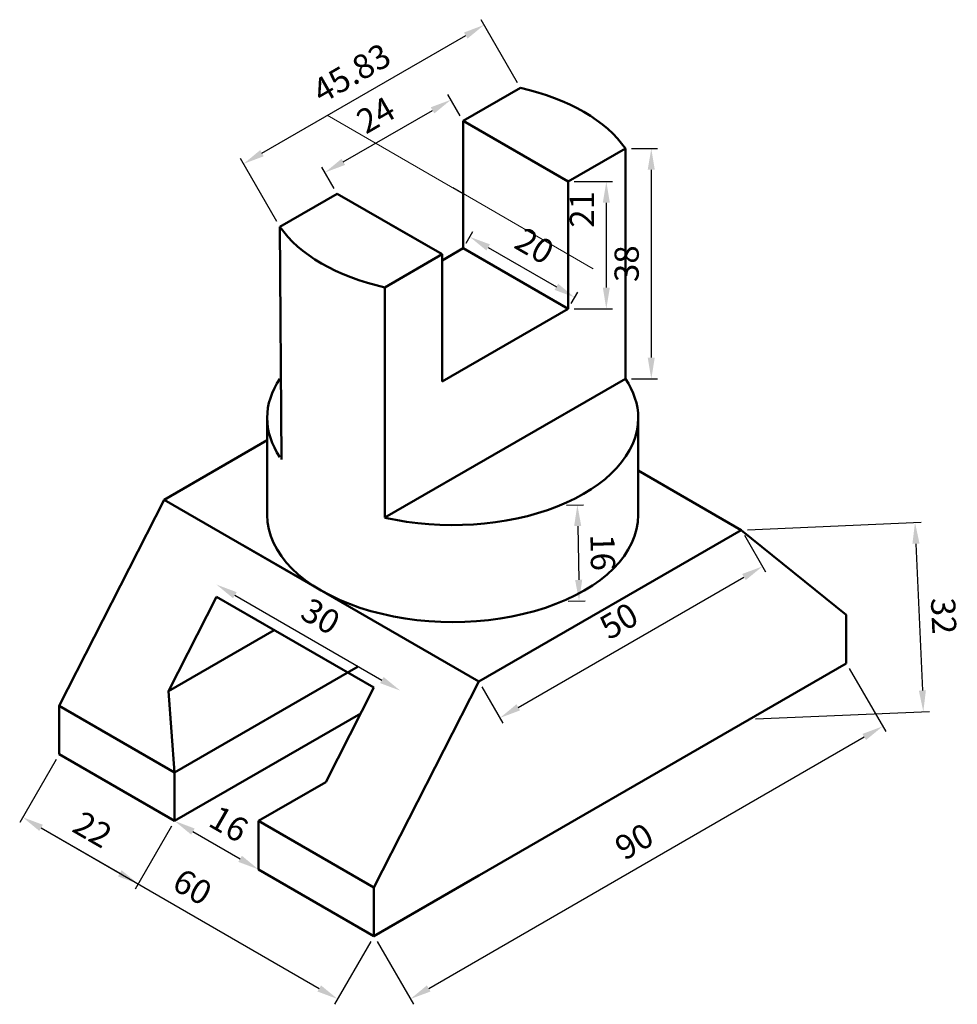
# Model space of a CAD drawing. Units: millimetres. Extents: x 3187 to 3342, y 774 to 936.
import ezdxf

# ---------------------------------------------------------------- set-up
doc = ezdxf.new("R2010")
doc.units = ezdxf.units.MM
doc.linetypes.add('CENTER', pattern=[50.8, 31.75, -6.35, 6.35, -6.35])
for name, color, linetype, lineweight in [('M-CNTR', 4, 'CENTER', 18), ('M-DIMS', 3, 'Continuous', 25), ('M-OUTL', 7, 'Continuous', 50)]:
    doc.layers.add(name, color=color, linetype=linetype, lineweight=lineweight)
doc.styles.get("Standard").update_dxf_attribs({"font": 'arial.ttf'})
doc.dimstyles.new('AM_ISO$0', dxfattribs={"dimtxt": 4, "dimasz": 3.5, "dimexe": 1, "dimexo": 1, "dimgap": 1.5, "dimtad": 1, "dimdsep": 46, "dimtxsty": 'Standard', "dimcen": 0, "dimclrd": 256, "dimclre": 256, "dimclrt": 2, "dimadec": 0, "dimazin": 2, "dimtp": 0.1, "dimtm": 0.1, "dimtfac": 0.71, "dimtmove": 0, "dimatfit": 3, "dimfxl": 1, "dimlwd": -1, "dimlwe": -1, "dimarcsym": 1})

# ---------------------------------------------------------------- blocks, each defined once
blk = doc.blocks.new('*D3')
at = {"layer": 'Defpoints', "color": 0, "transparency": 16777216}
for p in [(3323.73, 829.92), (3329.73, 819.53), (3245.79, 784.92)]:
    blk.add_point(p, dxfattribs=at)
at = {"layer": 'M-DIMS', "color": 0, "linetype": 'ByBlock', "transparency": 16777216}
for p, q in [((3324.23, 829.05), (3330.23, 818.66)), ((3254.82, 776.28), (3326.7, 817.78)), ((3246.29, 784.05), (3252.29, 773.66))]:
    blk.add_line(p, q, dxfattribs=at)
at = {"layer": 'M-DIMS', "color": 0, "transparency": 16777216}
for points in [[(3326.4, 818.28), (3326.99, 817.27), (3329.73, 819.53)], [(3254.52, 776.78), (3255.11, 775.77), (3251.79, 774.53)]]:
    blk.add_solid(points, dxfattribs=at)
at = {"layer": 'M-DIMS', "color": 0, "transparency": 16777216, "insert": (3288.99, 800.09), "char_height": 4, "attachment_point": 5, "rotation": 30}
blk.add_mtext('90', dxfattribs=at)
blk = doc.blocks.new('*D4')
at = {"layer": 'Defpoints', "color": 0, "transparency": 16777216}
for p in [(3306.41, 851.92), (3309.88, 845.91), (3263.11, 826.92)]:
    blk.add_point(p, dxfattribs=at)
at = {"layer": 'M-DIMS', "color": 0, "linetype": 'ByBlock', "transparency": 16777216}
for p, q in [((3306.91, 851.05), (3310.38, 845.05)), ((3269.6, 822.66), (3306.84, 844.16)), ((3263.61, 826.05), (3267.07, 820.05))]:
    blk.add_line(p, q, dxfattribs=at)
at = {"layer": 'M-DIMS', "color": 0, "transparency": 16777216}
for points in [[(3306.55, 844.67), (3307.14, 843.66), (3309.88, 845.91)], [(3269.31, 823.17), (3269.9, 822.16), (3266.57, 820.91)]]:
    blk.add_solid(points, dxfattribs=at)
at = {"layer": 'M-DIMS', "color": 0, "transparency": 16777216, "insert": (3286.45, 836.48), "char_height": 4, "attachment_point": 5, "rotation": 30}
blk.add_mtext('50', dxfattribs=at)
blk = doc.blocks.new('*D5')
at = {"layer": 'Defpoints', "color": 0, "transparency": 16777216}
for p in [(3193.82, 814.92), (3245.79, 784.92), (3239.79, 774.53)]:
    blk.add_point(p, dxfattribs=at)
at = {"layer": 'M-DIMS', "color": 0, "linetype": 'ByBlock', "transparency": 16777216}
for p, q in [((3193.32, 814.05), (3187.32, 803.66)), ((3190.85, 802.78), (3236.75, 776.28)), ((3245.29, 784.05), (3239.29, 773.66))]:
    blk.add_line(p, q, dxfattribs=at)
at = {"layer": 'M-DIMS', "color": 0, "transparency": 16777216}
for points in [[(3191.15, 803.28), (3190.56, 802.27), (3187.82, 804.53)], [(3237.05, 776.78), (3236.46, 775.77), (3239.79, 774.53)]]:
    blk.add_solid(points, dxfattribs=at)
at = {"layer": 'M-DIMS', "color": 0, "transparency": 16777216, "insert": (3215.58, 792.59), "char_height": 4, "attachment_point": 5, "rotation": 330}
blk.add_mtext('60', dxfattribs=at)
blk = doc.blocks.new('*D6')
at = {"layer": 'Defpoints', "color": 0, "transparency": 16777216}
for p in [(3193.82, 814.92), (3212.88, 803.92), (3206.88, 793.53)]:
    blk.add_point(p, dxfattribs=at)
at = {"layer": 'M-DIMS', "color": 0, "linetype": 'ByBlock', "transparency": 16777216}
for p, q in [((3193.32, 814.05), (3187.32, 803.66)), ((3190.85, 802.78), (3203.85, 795.28)), ((3212.38, 803.05), (3206.38, 792.66))]:
    blk.add_line(p, q, dxfattribs=at)
at = {"layer": 'M-DIMS', "color": 0, "transparency": 16777216}
for points in [[(3191.15, 803.28), (3190.56, 802.27), (3187.82, 804.53)], [(3204.14, 795.78), (3203.55, 794.77), (3206.88, 793.53)]]:
    blk.add_solid(points, dxfattribs=at)
at = {"layer": 'M-DIMS', "color": 0, "transparency": 16777216, "insert": (3199.1, 802.06), "char_height": 4, "attachment_point": 5, "rotation": 330}
blk.add_mtext('22', dxfattribs=at)
blk = doc.blocks.new('*D7')
at = {"layer": 'Defpoints', "color": 0, "transparency": 16777216}
for p in [(3212.88, 803.92), (3226.73, 795.92), (3226.73, 795.92)]:
    blk.add_point(p, dxfattribs=at)
at = {"layer": 'M-DIMS', "color": 0, "linetype": 'ByBlock', "transparency": 16777216}
blk.add_line((3215.91, 802.17), (3223.7, 797.67), dxfattribs=at)
at = {"layer": 'M-DIMS', "color": 0, "transparency": 16777216}
for points in [[(3216.2, 802.67), (3215.62, 801.66), (3212.88, 803.92)], [(3223.99, 798.17), (3223.41, 797.16), (3226.73, 795.92)]]:
    blk.add_solid(points, dxfattribs=at)
at = {"layer": 'M-DIMS', "color": 0, "transparency": 16777216, "insert": (3221.58, 802.99), "char_height": 4, "attachment_point": 5, "rotation": 330}
blk.add_mtext('16', dxfattribs=at)
blk = doc.blocks.new('*D8')
at = {"layer": 'Defpoints', "color": 0, "transparency": 16777216}
for p in [(3219.8, 842.92), (3250.12, 825.42), (3250.12, 825.42)]:
    blk.add_point(p, dxfattribs=at)
at = {"layer": 'M-DIMS', "color": 0, "linetype": 'ByBlock', "transparency": 16777216}
blk.add_line((3222.84, 841.17), (3247.08, 827.17), dxfattribs=at)
at = {"layer": 'M-DIMS', "color": 0, "transparency": 16777216}
for points in [[(3223.13, 841.67), (3222.54, 840.66), (3219.8, 842.92)], [(3247.38, 827.67), (3246.79, 826.66), (3250.12, 825.42)]]:
    blk.add_solid(points, dxfattribs=at)
at = {"layer": 'M-DIMS', "color": 0, "transparency": 16777216, "insert": (3236.73, 837.24), "char_height": 4, "attachment_point": 5, "rotation": 330}
blk.add_mtext('30', dxfattribs=at)
blk = doc.blocks.new('*D9')
at = {"layer": 'Defpoints', "color": 0, "transparency": 16777216}
for p in [(3276.56, 856.03), (3276.85, 840.15), (3279.63, 840.2)]:
    blk.add_point(p, dxfattribs=at)
at = {"layer": 'M-DIMS', "color": 0, "linetype": 'ByBlock', "transparency": 16777216}
for p, q in [((3277.56, 856.05), (3280.35, 856.1)), ((3279.41, 852.58), (3279.57, 843.7)), ((3277.85, 840.17), (3280.63, 840.22))]:
    blk.add_line(p, q, dxfattribs=at)
at = {"layer": 'M-DIMS', "color": 0, "transparency": 16777216}
for points in [[(3279.99, 852.59), (3278.82, 852.57), (3279.35, 856.08)], [(3280.15, 843.71), (3278.98, 843.69), (3279.63, 840.2)]]:
    blk.add_solid(points, dxfattribs=at)
at = {"layer": 'M-DIMS', "color": 0, "transparency": 16777216, "insert": (3283.03, 848.2), "char_height": 4, "attachment_point": 5, "rotation": 271.0309}
blk.add_mtext('16', dxfattribs=at)
blk = doc.blocks.new('*D10')
at = {"layer": 'Defpoints', "color": 0, "transparency": 16777216}
for p in [(3287.28, 914.87), (3287.28, 876.87), (3291.55, 876.87)]:
    blk.add_point(p, dxfattribs=at)
at = {"layer": 'M-DIMS', "color": 0, "linetype": 'ByBlock', "transparency": 16777216}
for p, q in [((3288.28, 914.87), (3292.55, 914.87)), ((3291.55, 911.37), (3291.55, 880.37)), ((3288.28, 876.87), (3292.55, 876.87))]:
    blk.add_line(p, q, dxfattribs=at)
at = {"layer": 'M-DIMS', "color": 0, "transparency": 16777216}
for points in [[(3290.96, 911.37), (3292.13, 911.37), (3291.55, 914.87)], [(3290.96, 880.37), (3292.13, 880.37), (3291.55, 876.87)]]:
    blk.add_solid(points, dxfattribs=at)
at = {"layer": 'M-DIMS', "color": 0, "transparency": 16777216, "insert": (3288, 895.87), "char_height": 4, "attachment_point": 5, "rotation": 90}
blk.add_mtext('38', dxfattribs=at)
blk = doc.blocks.new('*D11')
at = {"layer": 'Defpoints', "color": 0, "transparency": 16777216}
for p in [(3277.83, 909.42), (3277.83, 888.42), (3284.13, 888.42)]:
    blk.add_point(p, dxfattribs=at)
at = {"layer": 'M-DIMS', "color": 0, "linetype": 'ByBlock', "transparency": 16777216}
for p, q in [((3278.83, 909.42), (3285.13, 909.42)), ((3284.13, 905.92), (3284.13, 891.92)), ((3278.83, 888.42), (3285.13, 888.42))]:
    blk.add_line(p, q, dxfattribs=at)
at = {"layer": 'M-DIMS', "color": 0, "transparency": 16777216}
for points in [[(3283.55, 905.92), (3284.71, 905.92), (3284.13, 909.42)], [(3283.55, 891.92), (3284.71, 891.92), (3284.13, 888.42)]]:
    blk.add_solid(points, dxfattribs=at)
at = {"layer": 'M-DIMS', "color": 0, "transparency": 16777216, "insert": (3280.62, 904.83), "char_height": 4, "attachment_point": 5, "rotation": 90}
blk.add_mtext('21', dxfattribs=at)
blk = doc.blocks.new('*D12')
at = {"layer": 'Defpoints', "color": 0, "transparency": 16777216}
for p in [(3260.51, 898.42), (3278.92, 890.3), (3277.83, 888.42)]:
    blk.add_point(p, dxfattribs=at)
at = {"layer": 'M-DIMS', "color": 0, "linetype": 'ByBlock', "transparency": 16777216}
for p, q in [((3261.01, 899.28), (3262.1, 901.17)), ((3264.63, 898.55), (3275.89, 892.05)), ((3278.33, 889.28), (3279.42, 891.17))]:
    blk.add_line(p, q, dxfattribs=at)
at = {"layer": 'M-DIMS', "color": 0, "transparency": 16777216}
for points in [[(3264.92, 899.06), (3264.34, 898.05), (3261.6, 900.3)], [(3276.18, 892.56), (3275.59, 891.55), (3278.92, 890.3)]]:
    blk.add_solid(points, dxfattribs=at)
at = {"layer": 'M-DIMS', "color": 0, "transparency": 16777216, "insert": (3272.03, 898.37), "char_height": 4, "attachment_point": 5, "rotation": 330}
blk.add_mtext('20', dxfattribs=at)
blk = doc.blocks.new('*D13')
at = {"layer": 'Defpoints', "color": 0, "transparency": 16777216}
for p in [(3258.49, 922.92), (3260.51, 919.42), (3239.72, 907.42)]:
    blk.add_point(p, dxfattribs=at)
at = {"layer": 'M-DIMS', "color": 0, "linetype": 'ByBlock', "transparency": 16777216}
for p, q in [((3260.01, 920.28), (3257.99, 923.79)), ((3240.73, 912.67), (3255.45, 921.17)), ((3239.22, 908.28), (3237.2, 911.79))]:
    blk.add_line(p, q, dxfattribs=at)
at = {"layer": 'M-DIMS', "color": 0, "transparency": 16777216}
for points in [[(3255.16, 921.68), (3255.75, 920.67), (3258.49, 922.92)], [(3240.44, 913.18), (3241.02, 912.17), (3237.7, 910.92)]]:
    blk.add_solid(points, dxfattribs=at)
at = {"layer": 'M-DIMS', "color": 0, "transparency": 16777216, "insert": (3246.34, 919.96), "char_height": 4, "attachment_point": 5, "rotation": 30}
blk.add_mtext('24', dxfattribs=at)
blk = doc.blocks.new('*D14')
at = {"layer": 'Defpoints', "color": 0, "transparency": 16777216}
for p in [(3306.41, 851.92), (3307.77, 820.71), (3336.44, 821.96)]:
    blk.add_point(p, dxfattribs=at)
at = {"layer": 'M-DIMS', "color": 0, "linetype": 'ByBlock', "transparency": 16777216}
for p, q in [((3307.41, 851.96), (3336.07, 853.21)), ((3335.23, 849.67), (3336.28, 825.45)), ((3308.77, 820.75), (3337.44, 822))]:
    blk.add_line(p, q, dxfattribs=at)
at = {"layer": 'M-DIMS', "color": 0, "transparency": 16777216}
for points in [[(3335.81, 849.7), (3334.64, 849.65), (3335.07, 853.17)], [(3336.87, 825.48), (3335.7, 825.43), (3336.44, 821.96)]]:
    blk.add_solid(points, dxfattribs=at)
at = {"layer": 'M-DIMS', "color": 0, "transparency": 16777216, "insert": (3339.29, 837.72), "char_height": 4, "attachment_point": 5, "rotation": 272.5002}
blk.add_mtext('32', dxfattribs=at)
blk = doc.blocks.new('*D15')
at = {"layer": 'Defpoints', "color": 0, "transparency": 16777216}
for p in [(3263.96, 935.27), (3269.96, 924.87), (3230.27, 901.96)]:
    blk.add_point(p, dxfattribs=at)
at = {"layer": 'M-DIMS', "linetype": 'ByBlock', "transparency": 16777216}
for p, q in [((3269.46, 925.74), (3263.46, 936.13)), ((3227.3, 914.1), (3260.93, 933.52)), ((3229.77, 902.83), (3223.77, 913.22))]:
    blk.add_line(p, q, dxfattribs=at)
at = {"layer": 'M-DIMS', "transparency": 16777216}
for points in [[(3260.64, 934.02), (3261.22, 933.01), (3263.96, 935.27)], [(3227.01, 914.61), (3227.6, 913.6), (3224.27, 912.35)]]:
    blk.add_solid(points, dxfattribs=at)
at = {"layer": 'M-DIMS', "color": 2, "transparency": 16777216, "insert": (3242.34, 926.88), "char_height": 4, "attachment_point": 5, "rotation": 30}
blk.add_mtext('45.83', dxfattribs=at)

msp = doc.modelspace()

# ---------------------------------------------------------------- linework, layer by layer
at = {"layer": 'M-CNTR'}
for p, q in [((3260.508, 907.418), (3238.088, 920.362)), ((3258.776, 908.418), (3281.973, 895.025))]:
    msp.add_line(p, q, dxfattribs=at)
at = {"layer": 'M-OUTL'}
for p, q in [((3260.508, 919.418), (3269.959, 924.875)), ((3277.828, 909.418), (3260.508, 919.418)), ((3260.508, 919.418), (3260.508, 898.418)), ((3277.828, 909.418), (3287.279, 914.875)), ((3287.279, 914.875), (3287.279, 876.875)), ((3269.168, 914.418), (3277.828, 909.418)), ((3277.828, 909.418), (3277.828, 888.418)), ((3239.723, 907.418), (3230.272, 901.962)), ((3257.044, 897.418), (3239.723, 907.418)), ((3230.272, 901.962), (3230.553, 863.564)), ((3248.383, 902.418), (3257.044, 897.418)), ((3257.044, 897.418), (3247.593, 891.962)), ((3260.508, 898.418), (3257.044, 896.418)), ((3257.044, 897.418), (3257.044, 876.418)), ((3277.828, 888.418), (3260.508, 898.418)), ((3247.593, 891.962), (3247.593, 853.962)), ((3277.828, 888.418), (3257.044, 876.418)), ((3247.593, 853.962), (3287.279, 876.875)), ((3228.157, 854.418), (3228.157, 870.418)), ((3289.394, 854.418), (3289.394, 870.418)), ((3211.144, 856.918), (3228.157, 866.741)), ((3289.394, 861.741), (3306.407, 851.918)), ((3211.144, 856.918), (3193.824, 822.918)), ((3263.106, 826.918), (3211.144, 856.918)), ((3263.106, 826.918), (3306.407, 851.918)), ((3306.407, 851.918), (3323.728, 837.918)), ((3237.125, 841.918), (3224.135, 849.418)), ((3211.866, 825.335), (3219.805, 840.918)), ((3219.805, 840.918), (3245.785, 825.918)), ((3323.728, 829.918), (3323.728, 837.918)), ((3211.866, 825.335), (3229.331, 835.418)), ((3212.876, 811.918), (3243.187, 829.418)), ((3245.785, 784.918), (3323.728, 829.918)), ((3245.785, 825.918), (3237.847, 810.335)), ((3245.785, 792.918), (3263.106, 826.918)), ((3212.876, 811.918), (3211.866, 825.335)), ((3212.876, 811.918), (3193.824, 822.918)), ((3193.824, 822.918), (3193.824, 814.918)), ((3212.876, 803.918), (3243.62, 821.668)), ((3193.824, 814.918), (3212.876, 803.918)), ((3212.876, 803.918), (3212.876, 811.918)), ((3237.847, 810.335), (3226.733, 803.918)), ((3226.733, 803.918), (3226.733, 795.918)), ((3226.733, 803.918), (3245.785, 792.918)), ((3226.733, 795.918), (3245.785, 784.918)), ((3226.733, 795.918), (3245.785, 784.918)), ((3245.785, 784.918), (3263.106, 794.918)), ((3245.785, 784.918), (3245.785, 792.918))]:
    msp.add_line(p, q, dxfattribs=at)
for centre, major_axis, start_param, end_param in [((3258.776, 908.418), (-30.619, 0), 3.515474, 4.3385077), ((3258.776, 908.418), (-30.619, 0), 0.3738813, 1.196915), ((3258.776, 870.418), (30.619, 0), 2.7677113, 3.1415927), ((3258.776, 870.418), (30.619, 0), 0, 0.3738813), ((3258.776, 870.418), (30.619, 0), 3.1415927, 3.515474), ((3258.776, 870.418), (30.619, 0), 4.3385077, 6.2831853), ((3258.776, 854.418), (-30.619, 0), 6.2831853, 9.424778)]:
    msp.add_ellipse(centre, major_axis=major_axis, ratio=0.5773503, start_param=start_param, end_param=end_param, dxfattribs=at)

# ---------------------------------------------------------------- dimensions: what is measured, and where the dimension line sits
at = {"layer": 'M-DIMS'}
dim = msp.add_linear_dim(base=(3263.959, 935.267), p1=(3230.272, 901.962), p2=(3269.959, 924.875), angle=30, dimstyle='AM_ISO$0', override={"dimrnd": 0}, dxfattribs=at)
dim.commit()
dim.dimension.update_dxf_attribs({"geometry": '*D15', "text_midpoint": (3242.344, 926.879)})
for p1, p2, distance, override, picture, middle in [((3239.723, 907.418), (3260.508, 919.418), 4.044, {"dimclrd": 0, "dimclre": 0, "dimclrt": 0}, '*D13', (3246.339, 919.959)), ((3287.279, 914.875), (3287.279, 876.875), 4.269, {"dimclrd": 0, "dimclre": 0, "dimclrt": 0}, '*D10', (3288.005, 895.875)), ((3260.508, 898.418), (3277.828, 888.418), 2.178, {"dimclrd": 0, "dimclre": 0, "dimclrt": 0}, '*D12', (3272.028, 898.372)), ((3263.106, 826.918), (3306.407, 851.918), -6.936, {"dimclrd": 0, "dimclre": 0, "dimclrt": 0}, '*D4', (3286.453, 836.479)), ((3245.785, 784.918), (3323.728, 829.918), -12, {"dimpost": '', "dimclrd": 0, "dimclre": 0, "dimclrt": 0}, '*D3', (3288.985, 800.094)), ((3193.824, 814.918), (3245.785, 784.918), -12, {"dimpost": '', "dimclrd": 0, "dimclre": 0, "dimclrt": 0}, '*D5', (3215.576, 792.594)), ((3193.824, 814.918), (3212.876, 803.918), -12, {"dimclrd": 0, "dimclre": 0, "dimclrt": 0}, '*D6', (3199.104, 802.064)), ((3212.876, 803.918), (3226.733, 795.918), 0, {"dimclrd": 0, "dimclre": 0, "dimclrt": 0}, '*D7', (3221.576, 802.986))]:
    dim = msp.add_aligned_dim(p1=p1, p2=p2, distance=distance, dimstyle='AM_ISO$0', override=override, dxfattribs=at)
    dim.commit()
    dim.dimension.update_dxf_attribs({"geometry": picture, "text_midpoint": middle})
dim = msp.add_linear_dim(base=(3284.129, 888.418), p1=(3277.828, 909.418), p2=(3277.828, 888.418), angle=270, dimstyle='AM_ISO$0', override={"dimclrd": 0, "dimclre": 0, "dimclrt": 0}, dxfattribs=at)
dim.commit()
dim.dimension.update_dxf_attribs({"geometry": '*D11', "text_midpoint": (3284.129, 904.834), "dimtype": 161})
for p1, p2, distance, text, picture, middle in [((3276.56, 856.028), (3276.846, 840.147), 2.786, '16', '*D9', (3283.03, 848.202)), ((3306.407, 851.918), (3307.77, 820.705), 28.693, '32', '*D14', (3339.295, 837.718)), ((3219.805, 842.918), (3250.116, 825.418), 0, '30', '*D8', (3236.732, 837.237))]:
    dim = msp.add_aligned_dim(p1=p1, p2=p2, distance=distance, text=text, dimstyle='AM_ISO$0', override={"dimpost": '', "dimclrd": 0, "dimclre": 0, "dimclrt": 0}, dxfattribs=at)
    dim.commit()
    dim.dimension.update_dxf_attribs({"geometry": picture, "text_midpoint": middle})

doc.saveas('drawing.dxf')
